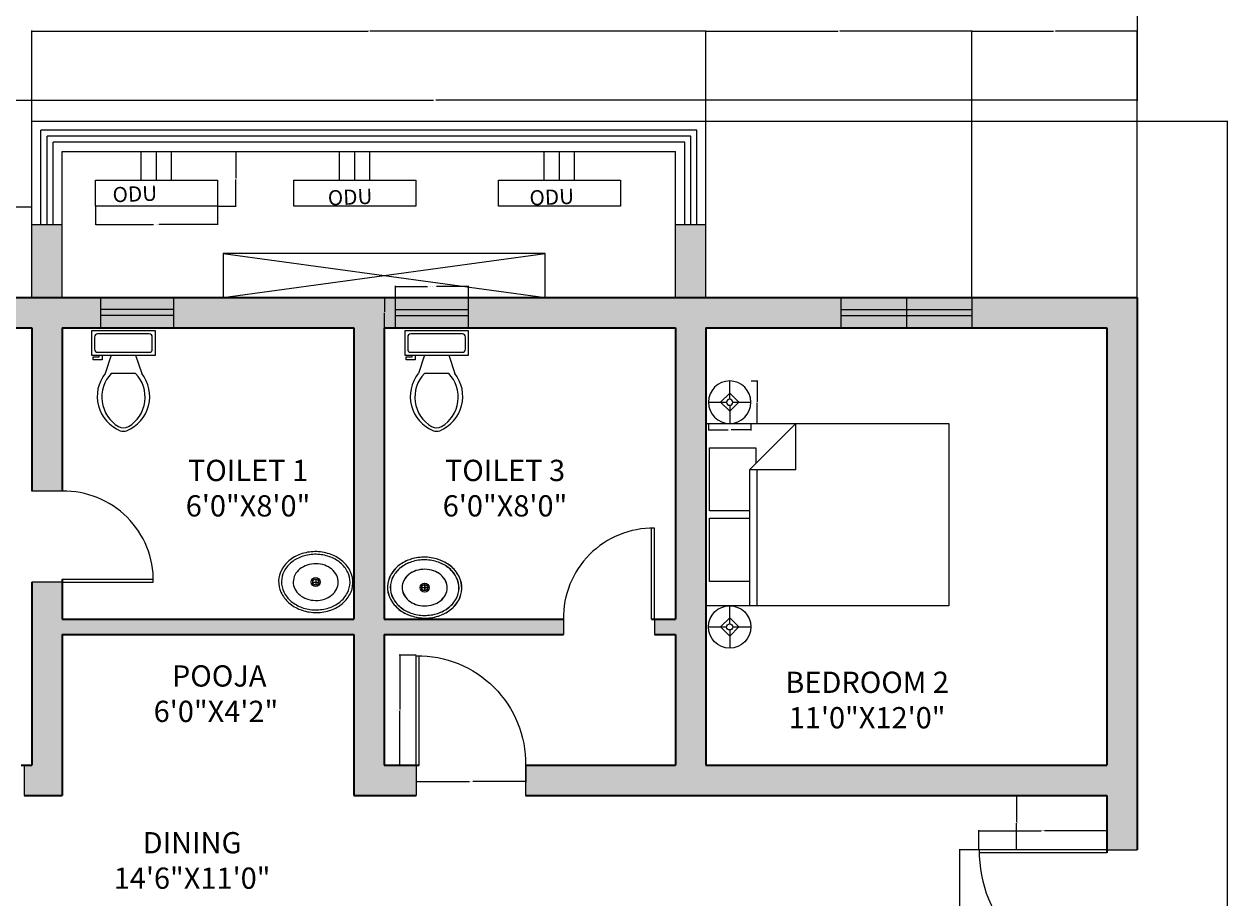
# Model space of a CAD drawing. Units: inches. Extents: x -382 to 250, y 518 to 1732.
# Tile 4 of 8: x -147 to 250, y 879 to 1167. Entities that reach past the tile are written whole.
import ezdxf

# ---------------------------------------------------------------- set-up
doc = ezdxf.new("R2010")
doc.units = ezdxf.units.IN
doc.header["$MEASUREMENT"] = 0
for name, color, linetype, lineweight in [('A-ANNO-DIMS', 2, 'Continuous', 18), ('A-AREA-IDEN', 7, 'Continuous', 18), ('A-DOOR', 3, 'Continuous', 18), ('A-FLOR-EDGE', 7, 'Continuous', 25), ('A-FLOR-FIXT', 8, 'Continuous', 18), ('A-FLOR-SHFT', 8, 'Continuous', 18), ('A-FURN', 8, 'Continuous', 18), ('A-GLAZ', 4, 'Continuous', 18), ('A-WALL', 7, 'Continuous', 35), ('M-ANNO-TEXT', 7, 'Continuous', 13), ('M-HVAC-EQPM', 4, 'Continuous', 18)]:
    doc.layers.add(name, color=color, linetype=linetype, lineweight=lineweight)
doc.layers.add('A-GLAZ-PATT', color=143, linetype='Continuous', lineweight=13, true_color=0x7aafdf)
doc.layers.add('A-WALL-PATT', color=251, linetype='Continuous', lineweight=13, true_color=0x636466)
doc.styles.get("Standard").update_dxf_attribs({"font": 'arial.ttf'})
doc.dimstyles.get("Standard").update_dxf_attribs({"dimtxt": 0.18, "dimasz": 0.18, "dimexe": 0.18, "dimexo": 0.0625, "dimgap": 0.09, "dimtad": 0, "dimtih": 1, "dimtoh": 1, "dimdec": 4, "dimzin": 0, "dimdsep": 46, "dimtxsty": 'Standard', "dimcen": 0.09, "dimadec": 0, "dimazin": 0, "dimtfac": 1, "dimtdec": 4, "dimtofl": 0, "dimtmove": 0, "dimatfit": 3, "dimfxl": 1, "dimtolj": 1, "dimtzin": 0, "dimarcsym": 0})

# ---------------------------------------------------------------- blocks, each defined once
blk = doc.blocks.new('Sink - Oval top')
for p, q in [((-1, 0), (1, 0)), ((0, 1), (0, -1))]:
    blk.add_line(p, q)
for points in [[(-12.23, 0.39, 0.117634), (-11.46, -3.36, 0.104469), (-8.88, -6.8, 0.090016), (-5.08, -9.07, 0.08192), (-0.32, -10.02, 0.08192), (4.49, -9.38, 0.090016), (8.42, -7.36, 0.104469), (11.22, -4.09, 0.117634), (12.23, -0.39, 0.117634), (11.46, 3.36, 0.104469), (8.88, 6.8, 0.090016), (5.08, 9.07, 0.08192), (0.32, 10.02, 0.08192), (-4.49, 9.38, 0.090016), (-8.42, 7.36, 0.104469), (-11.22, 4.09, 0.117634)], [(-11.29, 0.16, 0.118622), (-10.52, -3.25, 0.104678), (-8.07, -6.36, 0.089562), (-4.54, -8.37, 0.081185), (-0.13, -9.15, 0.081185), (4.3, -8.49, 0.089562), (7.89, -6.58, 0.104678), (10.42, -3.55, 0.118622), (11.29, -0.16, 0.118622), (10.52, 3.25, 0.104678), (8.07, 6.36, 0.089562), (4.54, 8.37, 0.081185), (0.13, 9.15, 0.081185), (-4.3, 8.49, 0.089562), (-7.89, 6.58, 0.104678), (-10.42, 3.55, 0.118622)], [(-7.42, 0.08, 0.118283), (-6.91, -2.17, 0.104607), (-5.29, -4.21, 0.089718), (-2.97, -5.53, 0.081436), (-0.07, -6.04, 0.081436), (2.84, -5.59, 0.089718), (5.2, -4.33, 0.104607), (6.86, -2.32, 0.118283), (7.42, -0.08, 0.118283), (6.91, 2.17, 0.104607), (5.29, 4.21, 0.089718), (2.97, 5.53, 0.081436), (0.07, 6.04, 0.081436), (-2.84, 5.59, 0.089718), (-5.2, 4.33, 0.104607), (-6.86, 2.32, 0.118283)]]:
    blk.add_lwpolyline(points, format="xyb", close=True)
for radius in [1.5, 1]:
    blk.add_circle((0, 0), radius)
blk = doc.blocks.new('Bed - Queen')
for p, q in [((0, -80.00003), (0, 0)), ((0, 0), (59.99999, 0)), ((59.99999, 0), (59.99999, -80.00003)), ((7.99999, -1.2), (28.79998, -1.2)), ((7.99999, -14.4), (7.99999, -1.2)), ((28.79998, -1.2), (28.79998, -14.4)), ((31.19999, -1.2), (51.99999, -1.2)), ((31.19999, -14.4), (31.19999, -1.2)), ((51.99999, -1.2), (51.99999, -16.4)), ((0, -14.4), (44.8, -14.4)), ((59.99999, -29.6), (44.8, -14.4)), ((44.8, -14.4), (44.8, -29.6)), ((44.8, -16.8), (0, -16.8)), ((51.99999, -16.4), (46.79936, -16.4)), ((44.8, -29.6), (59.99999, -29.6)), ((59.99999, -80.00003), (0, -80.00003))]:
    blk.add_line(p, q)
blk = doc.blocks.new('Lamp - Table')
for p, q in [((0, 7), (0, 1)), ((-1, 0), (-7, 0)), ((0, 3), (-3, 0)), ((-3, 0), (0, -3)), ((3, 0), (0, 3)), ((0, -3), (3, 0)), ((1, 0), (7, 0)), ((0, -1), (0, -7))]:
    blk.add_line(p, q)
for radius in [7, 1]:
    blk.add_circle((0, 0), radius)
blk = doc.blocks.new('Toilet - top')
for p, q in [((9.5, -6), (9.5, -2)), ((-10, -8.5), (-8, -8.5)), ((-10, -9.5), (-10, -8.5)), ((-7, -9.5), (-10, -9.5)), ((-8, -8.5), (-8, -8)), ((-7, -8), (-7, -9.5)), ((-4, -8), (-6, -14)), ((4, -8), (6, -14)), ((4, -14), (-4, -14))]:
    blk.add_line(p, q)
blk.add_lwpolyline([(10.5, -8), (10.5, 0), (-10.5, 0), (-10.5, -8)], close=True)
for points in [[(-9.5, -2), (-9.5, -6)], [(8.5, -1), (-8.5, -1)], [(-8.5, -7), (8.5, -7)]]:
    blk.add_lwpolyline(points)
for centre, radius, start, end in [((-8.62, -1.88), 0.884, 81.8699, 188.1301), ((8.62, -1.88), 0.884, 351.8699, 98.1301), ((-8.62, -6.12), 0.884, 171.8699, 278.1301), ((8.62, -6.12), 0.884, 261.8699, 8.1301), ((3.52, -21.58), 12.17, 141.4691, 247.9714), ((4.2, -21.82), 11.33, 136.3677, 238.9468), ((-3.52, -21.58), 12.17, 292.0284, 38.5307), ((-4.2, -21.82), 11.33, 301.053, 43.6321), ((0, -27.88), 4, 245.7318, 294.2682), ((0, -29), 4, 254.8605, 285.1395)]:
    blk.add_arc(centre, radius, start, end)
blk = doc.blocks.new('WIN-24IN')
for p, q in [((0, 0), (0, 10)), ((24, 0), (24, 10)), ((0, 6), (24, 6)), ((0, 4), (24, 4))]:
    blk.add_line(p, q)
blk = doc.blocks.new('DOOR-SWING-36IN')
for p, q in [((-1, 0), (-1, 36)), ((0, 0), (0, 36))]:
    blk.add_line(p, q)
blk.add_arc((-0.5, 0.5), 35.5, 89.1931, 180.8069)
blk = doc.blocks.new('DOOR-SWING-30IN')
for p, q in [((0, 1), (30, 1)), ((0, 0), (30, 0))]:
    blk.add_line(p, q)
blk.add_arc((0.5, 0.5), 29.5, 359.029, 90.971)
blk = doc.blocks.new('ODU-LEDGE-LARGE')
for p, q in [((15.1, 8.56), (15.1, 17.94)), ((20.1, 8.56), (20.1, 17.94)), ((25.1, 8.56), (25.1, 17.94))]:
    blk.add_line(p, q)
blk.add_lwpolyline([(0, 8.56), (40.21, 8.56), (40.21, 0), (0, 0)], close=True)
blk = doc.blocks.new('DOOR-ENTRY-42IN')
for p, q in [((0, 0), (-42, 0)), ((0, -1), (-42, -1))]:
    blk.add_line(p, q)
blk.add_arc((-0.5, -0.5), 41.5, 179.3097, 270.6903)
blk = doc.blocks.new('*D30')
at = {"layer": 'A-ANNO-DIMS', "color": 0, "lineweight": -2, "transparency": 16777216}
for p, q in [((92.66, 1049.55), (94.88, 1049.55)), ((94.7, 1049.37), (94.7, 1042.73)), ((94.7, 1035.73), (94.7, 1042.37)), ((92.66, 1035.55), (94.88, 1035.55))]:
    blk.add_line(p, q, dxfattribs=at)
at = {"layer": 'A-ANNO-DIMS', "color": 0, "transparency": 16777216}
for points in [[(94.67, 1049.37), (94.73, 1049.37), (94.7, 1049.55)], [(94.67, 1035.73), (94.73, 1035.73), (94.7, 1035.55)]]:
    blk.add_solid(points, dxfattribs=at)
at = {"layer": 'Defpoints', "color": 0, "transparency": 16777216}
for p in [(92.6, 1049.55), (92.6, 1035.55), (94.7, 1035.55)]:
    blk.add_point(p, dxfattribs=at)
at = {"layer": 'A-ANNO-DIMS', "color": 0, "transparency": 16777216, "insert": (94.7, 1042.55), "char_height": 0.18, "attachment_point": 5}
blk.add_mtext('\\A1;LAMP 14 TYP.', dxfattribs=at)
blk = doc.blocks.new('*D31')
at = {"layer": 'A-ANNO-DIMS', "color": 0, "lineweight": -2, "transparency": 16777216}
for p, q in [((78.6, 1035.49), (78.6, 1033.27)), ((92.6, 1035.49), (92.6, 1033.27)), ((78.78, 1033.45), (85.08, 1033.45)), ((92.42, 1033.45), (86.12, 1033.45))]:
    blk.add_line(p, q, dxfattribs=at)
at = {"layer": 'A-ANNO-DIMS', "color": 0, "transparency": 16777216}
for points in [[(78.78, 1033.48), (78.78, 1033.42), (78.6, 1033.45)], [(92.42, 1033.48), (92.42, 1033.42), (92.6, 1033.45)]]:
    blk.add_solid(points, dxfattribs=at)
at = {"layer": 'Defpoints', "color": 0, "transparency": 16777216}
for p in [(78.6, 1035.55), (92.6, 1035.55), (78.6, 1033.45)]:
    blk.add_point(p, dxfattribs=at)
at = {"layer": 'A-ANNO-DIMS', "color": 0, "transparency": 16777216, "insert": (85.6, 1033.45), "char_height": 0.18, "attachment_point": 5}
blk.add_mtext('\\A1;14 TYP.', dxfattribs=at)
blk = doc.blocks.new('*D50')
at = {"layer": 'A-ANNO-DIMS', "color": 0, "lineweight": -2, "transparency": 16777216}
for p, q in [((-123.3, 1107.06), (-123.3, 1100.92)), ((-83.09, 1107.06), (-83.09, 1100.92)), ((-123.12, 1101.1), (-104.15, 1101.1)), ((-83.27, 1101.1), (-102.24, 1101.1))]:
    blk.add_line(p, q, dxfattribs=at)
at = {"layer": 'A-ANNO-DIMS', "color": 0, "transparency": 16777216}
for points in [[(-123.12, 1101.13), (-123.12, 1101.07), (-123.3, 1101.1)], [(-83.27, 1101.13), (-83.27, 1101.07), (-83.09, 1101.1)]]:
    blk.add_solid(points, dxfattribs=at)
at = {"layer": 'Defpoints', "color": 0, "transparency": 16777216}
for p in [(-123.3, 1107.13), (-83.09, 1107.13), (-83.09, 1101.1)]:
    blk.add_point(p, dxfattribs=at)
at = {"layer": 'A-ANNO-DIMS', "color": 0, "transparency": 16777216, "insert": (-103.2, 1101.1), "char_height": 0.18, "attachment_point": 5}
blk.add_mtext('\\A1;ODU-L 40 TYP.', dxfattribs=at)
blk = doc.blocks.new('*D51')
at = {"layer": 'A-ANNO-DIMS', "color": 0, "lineweight": -2, "transparency": 16777216}
for p, q in [((-83.03, 1125.07), (-76.88, 1125.07)), ((-77.06, 1124.89), (-77.06, 1116.28)), ((-77.06, 1107.31), (-77.06, 1115.92)), ((-83.03, 1107.13), (-76.88, 1107.13))]:
    blk.add_line(p, q, dxfattribs=at)
at = {"layer": 'A-ANNO-DIMS', "color": 0, "transparency": 16777216}
for points in [[(-77.09, 1124.89), (-77.03, 1124.89), (-77.06, 1125.07)], [(-77.09, 1107.31), (-77.03, 1107.31), (-77.06, 1107.13)]]:
    blk.add_solid(points, dxfattribs=at)
at = {"layer": 'Defpoints', "color": 0, "transparency": 16777216}
for p in [(-83.09, 1125.07), (-77.06, 1125.07), (-83.09, 1107.13)]:
    blk.add_point(p, dxfattribs=at)
at = {"layer": 'A-ANNO-DIMS', "color": 0, "transparency": 16777216, "insert": (-77.06, 1116.1), "char_height": 0.18, "attachment_point": 5}
blk.add_mtext('\\A1;18 TYP.', dxfattribs=at)
blk = doc.blocks.new('*D58')
at = {"layer": 'A-ANNO-DIMS', "color": 0, "lineweight": -2, "transparency": 16777216}
for p, q in [((167.59, 895.12), (161.15, 895.12)), ((161.33, 894.94), (161.33, 874.24)), ((161.33, 853.17), (161.33, 873.87)), ((167.59, 852.99), (161.15, 852.99))]:
    blk.add_line(p, q, dxfattribs=at)
at = {"layer": 'A-ANNO-DIMS', "color": 0, "transparency": 16777216}
for points in [[(161.3, 894.94), (161.36, 894.94), (161.33, 895.12)], [(161.3, 853.17), (161.36, 853.17), (161.33, 852.99)]]:
    blk.add_solid(points, dxfattribs=at)
at = {"layer": 'Defpoints', "color": 0, "transparency": 16777216}
for p in [(161.33, 895.12), (167.65, 895.12), (167.65, 852.99)]:
    blk.add_point(p, dxfattribs=at)
at = {"layer": 'A-ANNO-DIMS', "color": 0, "transparency": 16777216, "insert": (161.33, 874.06), "char_height": 0.18, "attachment_point": 5}
blk.add_mtext('\\A1;ENTRY DOOR 42 TYP.', dxfattribs=at)
blk = doc.blocks.new('*D59')
at = {"layer": 'A-ANNO-DIMS', "color": 0, "lineweight": -2, "transparency": 16777216}
for p, q in [((167.65, 895.19), (167.65, 901.62)), ((167.83, 901.44), (188.19, 901.44)), ((209.6, 901.44), (189.25, 901.44)), ((209.78, 895.19), (209.78, 901.62))]:
    blk.add_line(p, q, dxfattribs=at)
at = {"layer": 'A-ANNO-DIMS', "color": 0, "transparency": 16777216}
for points in [[(167.83, 901.47), (167.83, 901.41), (167.65, 901.44)], [(209.6, 901.47), (209.6, 901.41), (209.78, 901.44)]]:
    blk.add_solid(points, dxfattribs=at)
at = {"layer": 'Defpoints', "color": 0, "transparency": 16777216}
for p in [(209.78, 901.44), (167.65, 895.12), (209.78, 895.12)]:
    blk.add_point(p, dxfattribs=at)
at = {"layer": 'A-ANNO-DIMS', "color": 0, "transparency": 16777216, "insert": (188.72, 901.44), "char_height": 0.18, "attachment_point": 5}
blk.add_mtext('\\A1;42 TYP.', dxfattribs=at)
blk = doc.blocks.new('*D60')
at = {"layer": 'A-ANNO-DIMS', "color": 0, "lineweight": -2, "transparency": 16777216}
for p, q in [((-17.69, 959.2), (-23.22, 959.2)), ((-23.04, 959.02), (-23.04, 941.32)), ((-23.04, 923.25), (-23.04, 940.95)), ((-17.69, 923.07), (-23.22, 923.07))]:
    blk.add_line(p, q, dxfattribs=at)
at = {"layer": 'A-ANNO-DIMS', "color": 0, "transparency": 16777216}
for points in [[(-23.07, 959.02), (-23.01, 959.02), (-23.04, 959.2)], [(-23.07, 923.25), (-23.01, 923.25), (-23.04, 923.07)]]:
    blk.add_solid(points, dxfattribs=at)
at = {"layer": 'Defpoints', "color": 0, "transparency": 16777216}
for p in [(-23.04, 959.2), (-17.62, 959.2), (-17.62, 923.07)]:
    blk.add_point(p, dxfattribs=at)
at = {"layer": 'A-ANNO-DIMS', "color": 0, "transparency": 16777216, "insert": (-23.04, 941.14), "char_height": 0.18, "attachment_point": 5}
blk.add_mtext('\\A1;ROOM DOOR 36 TYP.', dxfattribs=at)
blk = doc.blocks.new('*D61')
at = {"layer": 'A-ANNO-DIMS', "color": 0, "lineweight": -2, "transparency": 16777216}
for p, q in [((-17.62, 923.01), (-17.62, 917.47)), ((18.51, 923.01), (18.51, 917.47)), ((-17.44, 917.65), (-0.08, 917.65)), ((18.33, 917.65), (0.97, 917.65))]:
    blk.add_line(p, q, dxfattribs=at)
at = {"layer": 'A-ANNO-DIMS', "color": 0, "transparency": 16777216}
for points in [[(-17.44, 917.68), (-17.44, 917.62), (-17.62, 917.65)], [(18.33, 917.68), (18.33, 917.62), (18.51, 917.65)]]:
    blk.add_solid(points, dxfattribs=at)
at = {"layer": 'Defpoints', "color": 0, "transparency": 16777216}
for p in [(-17.62, 923.07), (18.51, 923.07), (-17.62, 917.65)]:
    blk.add_point(p, dxfattribs=at)
at = {"layer": 'A-ANNO-DIMS', "color": 0, "transparency": 16777216, "insert": (0.44, 917.65), "char_height": 0.18, "attachment_point": 5}
blk.add_mtext('\\A1;36 TYP.', dxfattribs=at)
blk = doc.blocks.new('*D72')
at = {"layer": 'A-ANNO-DIMS', "color": 0, "lineweight": -2, "transparency": 16777216}
for p, q in [((-24.44, 1077.13), (-24.44, 1080.85)), ((-24.26, 1080.67), (-13.93, 1080.67)), ((-0.62, 1080.67), (-10.95, 1080.67)), ((-0.44, 1077.13), (-0.44, 1080.85))]:
    blk.add_line(p, q, dxfattribs=at)
at = {"layer": 'A-ANNO-DIMS', "color": 0, "transparency": 16777216}
for points in [[(-24.26, 1080.7), (-24.26, 1080.64), (-24.44, 1080.67)], [(-0.62, 1080.7), (-0.62, 1080.64), (-0.44, 1080.67)]]:
    blk.add_solid(points, dxfattribs=at)
at = {"layer": 'Defpoints', "color": 0, "transparency": 16777216}
for p in [(-0.44, 1080.67), (-24.44, 1077.07), (-0.44, 1077.07)]:
    blk.add_point(p, dxfattribs=at)
at = {"layer": 'A-ANNO-DIMS', "color": 0, "transparency": 16777216, "insert": (-12.44, 1080.67), "char_height": 0.18, "attachment_point": 5}
blk.add_mtext('\\A1;VENT WINDOW 24 TYP.', dxfattribs=at)
blk = doc.blocks.new('*D73')
at = {"layer": 'A-ANNO-DIMS', "color": 0, "lineweight": -2, "transparency": 16777216}
for p, q in [((-24.5, 1077.07), (-28.22, 1077.07)), ((-28.04, 1076.89), (-28.04, 1072.25)), ((-28.04, 1067.25), (-28.04, 1071.89)), ((-24.5, 1067.07), (-28.22, 1067.07))]:
    blk.add_line(p, q, dxfattribs=at)
at = {"layer": 'A-ANNO-DIMS', "color": 0, "transparency": 16777216}
for points in [[(-28.07, 1076.89), (-28.01, 1076.89), (-28.04, 1077.07)], [(-28.07, 1067.25), (-28.01, 1067.25), (-28.04, 1067.07)]]:
    blk.add_solid(points, dxfattribs=at)
at = {"layer": 'Defpoints', "color": 0, "transparency": 16777216}
for p in [(-28.04, 1077.07), (-24.44, 1077.07), (-24.44, 1067.07)]:
    blk.add_point(p, dxfattribs=at)
at = {"layer": 'A-ANNO-DIMS', "color": 0, "transparency": 16777216, "insert": (-28.04, 1072.07), "char_height": 0.18, "attachment_point": 5}
blk.add_mtext('\\A1;10 TYP.', dxfattribs=at)
blk = doc.blocks.new('*D75')
at = {"layer": 'A-ANNO-DIMS', "color": 0, "lineweight": -2, "transparency": 16777216}
for p, q in [((77.85, 1135.07), (249.66, 1135.07)), ((249.48, 1134.89), (249.48, 841.75)), ((249.48, 548.25), (249.48, 841.39)), ((58.85, 548.07), (249.66, 548.07))]:
    blk.add_line(p, q, dxfattribs=at)
at = {"layer": 'A-ANNO-DIMS', "color": 0, "transparency": 16777216}
for points in [[(249.45, 1134.89), (249.51, 1134.89), (249.48, 1135.07)], [(249.45, 548.25), (249.51, 548.25), (249.48, 548.07)]]:
    blk.add_solid(points, dxfattribs=at)
at = {"layer": 'Defpoints', "color": 0, "transparency": 16777216}
for p in [(77.78, 1135.07), (249.48, 1135.07), (58.78, 548.07)]:
    blk.add_point(p, dxfattribs=at)
at = {"layer": 'A-ANNO-DIMS', "color": 0, "transparency": 16777216, "insert": (249.48, 841.57), "char_height": 0.18, "attachment_point": 5}
blk.add_mtext('\\A1;587', dxfattribs=at)
blk = doc.blocks.new('*D76')
at = {"layer": 'A-ANNO-DIMS', "color": 0, "lineweight": -2, "transparency": 16777216}
for p, q in [((-298.22, 1077.13), (-298.22, 1106.95)), ((-298.04, 1106.77), (-221.5, 1106.77)), ((-144.4, 1106.77), (-220.94, 1106.77)), ((-144.22, 1077.13), (-144.22, 1106.95))]:
    blk.add_line(p, q, dxfattribs=at)
at = {"layer": 'A-ANNO-DIMS', "color": 0, "transparency": 16777216}
for points in [[(-298.04, 1106.8), (-298.04, 1106.74), (-298.22, 1106.77)], [(-144.4, 1106.8), (-144.4, 1106.74), (-144.22, 1106.77)]]:
    blk.add_solid(points, dxfattribs=at)
at = {"layer": 'Defpoints', "color": 0, "transparency": 16777216}
for p in [(-144.22, 1106.77), (-298.22, 1077.07), (-144.22, 1077.07)]:
    blk.add_point(p, dxfattribs=at)
at = {"layer": 'A-ANNO-DIMS', "color": 0, "transparency": 16777216, "insert": (-221.22, 1106.77), "char_height": 0.18, "attachment_point": 5}
blk.add_mtext('\\A1;154', dxfattribs=at)
blk = doc.blocks.new('*D77')
at = {"layer": 'A-ANNO-DIMS', "color": 0, "lineweight": -2, "transparency": 16777216}
for p, q in [((-144.22, 1135.13), (-144.22, 1164.95)), ((-144.04, 1164.77), (-33.5, 1164.77)), ((77.6, 1164.77), (-32.93, 1164.77)), ((77.78, 1135.13), (77.78, 1164.95))]:
    blk.add_line(p, q, dxfattribs=at)
at = {"layer": 'A-ANNO-DIMS', "color": 0, "transparency": 16777216}
for points in [[(-144.04, 1164.8), (-144.04, 1164.74), (-144.22, 1164.77)], [(77.6, 1164.8), (77.6, 1164.74), (77.78, 1164.77)]]:
    blk.add_solid(points, dxfattribs=at)
at = {"layer": 'Defpoints', "color": 0, "transparency": 16777216}
for p in [(77.78, 1164.77), (-144.22, 1135.07), (77.78, 1135.07)]:
    blk.add_point(p, dxfattribs=at)
at = {"layer": 'A-ANNO-DIMS', "color": 0, "transparency": 16777216, "insert": (-33.22, 1164.77), "char_height": 0.18, "attachment_point": 5}
blk.add_mtext('\\A1;222', dxfattribs=at)
blk = doc.blocks.new('*D78')
at = {"layer": 'A-ANNO-DIMS', "color": 0, "lineweight": -2, "transparency": 16777216}
for p, q in [((77.78, 1135.13), (77.78, 1164.95)), ((77.96, 1164.77), (121.26, 1164.77)), ((165.2, 1164.77), (121.91, 1164.77)), ((165.38, 1077.13), (165.38, 1164.95))]:
    blk.add_line(p, q, dxfattribs=at)
at = {"layer": 'A-ANNO-DIMS', "color": 0, "transparency": 16777216}
for points in [[(77.96, 1164.8), (77.96, 1164.74), (77.78, 1164.77)], [(165.2, 1164.8), (165.2, 1164.74), (165.38, 1164.77)]]:
    blk.add_solid(points, dxfattribs=at)
at = {"layer": 'Defpoints', "color": 0, "transparency": 16777216}
for p in [(165.38, 1164.77), (77.78, 1135.07), (165.38, 1077.07)]:
    blk.add_point(p, dxfattribs=at)
at = {"layer": 'A-ANNO-DIMS', "color": 0, "transparency": 16777216, "insert": (121.58, 1164.77), "char_height": 0.18, "attachment_point": 5}
blk.add_mtext('\\A1;87.6', dxfattribs=at)
blk = doc.blocks.new('*D83')
at = {"layer": 'A-ANNO-DIMS', "color": 0, "lineweight": -2, "transparency": 16777216}
for p, q in [((209.72, 913.07), (179.9, 913.07)), ((180.08, 912.89), (180.08, 904.28)), ((180.08, 895.3), (180.08, 903.91)), ((209.72, 895.12), (179.9, 895.12))]:
    blk.add_line(p, q, dxfattribs=at)
at = {"layer": 'A-ANNO-DIMS', "color": 0, "transparency": 16777216}
for points in [[(180.05, 912.89), (180.11, 912.89), (180.08, 913.07)], [(180.05, 895.3), (180.11, 895.3), (180.08, 895.12)]]:
    blk.add_solid(points, dxfattribs=at)
at = {"layer": 'Defpoints', "color": 0, "transparency": 16777216}
for p in [(180.08, 913.07), (209.78, 913.07), (209.78, 895.12)]:
    blk.add_point(p, dxfattribs=at)
at = {"layer": 'A-ANNO-DIMS', "color": 0, "transparency": 16777216, "insert": (180.08, 904.1), "char_height": 0.18, "attachment_point": 5}
blk.add_mtext('\\A1;17.945', dxfattribs=at)
blk = doc.blocks.new('*D84')
at = {"layer": 'A-ANNO-DIMS', "color": 0, "lineweight": -2, "transparency": 16777216}
for p, q in [((165.38, 1077.13), (165.38, 1164.95)), ((165.56, 1164.77), (192.26, 1164.77)), ((219.6, 1164.77), (192.91, 1164.77)), ((219.78, 1077.13), (219.78, 1164.95))]:
    blk.add_line(p, q, dxfattribs=at)
at = {"layer": 'A-ANNO-DIMS', "color": 0, "transparency": 16777216}
for points in [[(165.56, 1164.8), (165.56, 1164.74), (165.38, 1164.77)], [(219.6, 1164.8), (219.6, 1164.74), (219.78, 1164.77)]]:
    blk.add_solid(points, dxfattribs=at)
at = {"layer": 'Defpoints', "color": 0, "transparency": 16777216}
for p in [(219.78, 1164.77), (165.38, 1077.07), (219.78, 1077.07)]:
    blk.add_point(p, dxfattribs=at)
at = {"layer": 'A-ANNO-DIMS', "color": 0, "transparency": 16777216, "insert": (192.58, 1164.77), "char_height": 0.18, "attachment_point": 5}
blk.add_mtext('\\A1;54.4', dxfattribs=at)
blk = doc.blocks.new('*D86')
at = {"layer": 'A-ANNO-DIMS', "color": 0, "lineweight": -2, "transparency": 16777216}
for p, q in [((-242.98, 1352.01), (-242.98, 1141.82)), ((219.78, 1197.01), (219.78, 1141.82)), ((-242.8, 1142), (-11.99, 1142)), ((219.6, 1142), (-11.2, 1142))]:
    blk.add_line(p, q, dxfattribs=at)
at = {"layer": 'A-ANNO-DIMS', "color": 0, "transparency": 16777216}
for points in [[(-242.8, 1142.03), (-242.8, 1141.97), (-242.98, 1142)], [(219.6, 1142.03), (219.6, 1141.97), (219.78, 1142)]]:
    blk.add_solid(points, dxfattribs=at)
at = {"layer": 'Defpoints', "color": 0, "transparency": 16777216}
for p in [(-242.98, 1352.07), (219.78, 1197.07), (219.78, 1142)]:
    blk.add_point(p, dxfattribs=at)
at = {"layer": 'A-ANNO-DIMS', "color": 0, "transparency": 16777216, "insert": (-11.6, 1142), "char_height": 0.18, "attachment_point": 5}
blk.add_mtext('\\A1;462.8', dxfattribs=at)

msp = doc.modelspace()

# ---------------------------------------------------------------- hatches: boundary and pattern name
at = {"layer": 'A-GLAZ-PATT'}
h = msp.add_hatch(color=256, dxfattribs=at)
h.dxf.hatch_style = 1
h.paths.add_polyline_path([(-97.6147, 1077.0687), (-121.6147, 1077.0687), (-121.6147, 1073.0687), (-97.6147, 1073.0687)])
h = msp.add_hatch(color=256, dxfattribs=at)
h.dxf.hatch_style = 1
h.paths.add_polyline_path([(-0.4384, 1077.0687), (-24.4384, 1077.0687), (-24.4384, 1073.0687), (-0.4384, 1073.0687)])
h = msp.add_hatch(color=256, dxfattribs=at)
h.dxf.hatch_style = 1
h.paths.add_polyline_path([(143.785, 1077.0687), (122.185, 1077.0687), (122.185, 1073.0687), (143.785, 1073.0687)])
h = msp.add_hatch(color=256, dxfattribs=at)
h.dxf.hatch_style = 1
h.paths.add_polyline_path([(165.385, 1077.0687), (143.785, 1077.0687), (143.785, 1073.0687), (165.385, 1073.0687)])
h = msp.add_hatch(color=256, dxfattribs=at)
h.dxf.hatch_style = 1
h.paths.add_polyline_path([(-97.6147, 1073.0687), (-121.6147, 1073.0687), (-121.6147, 1071.0687), (-97.6147, 1071.0687)])
h = msp.add_hatch(color=256, dxfattribs=at)
h.dxf.hatch_style = 1
h.paths.add_polyline_path([(-97.6147, 1071.0687), (-121.6147, 1071.0687), (-121.6147, 1067.0687), (-97.6147, 1067.0687)])
h = msp.add_hatch(color=256, dxfattribs=at)
h.dxf.hatch_style = 1
h.paths.add_polyline_path([(-0.4384, 1073.0687), (-24.4384, 1073.0687), (-24.4384, 1071.0687), (-0.4384, 1071.0687)])
h = msp.add_hatch(color=256, dxfattribs=at)
h.dxf.hatch_style = 1
h.paths.add_polyline_path([(-0.4384, 1071.0687), (-24.4384, 1071.0687), (-24.4384, 1067.0687), (-0.4384, 1067.0687)])
h = msp.add_hatch(color=256, dxfattribs=at)
h.dxf.hatch_style = 1
h.paths.add_polyline_path([(143.785, 1073.0687), (122.185, 1073.0687), (122.185, 1071.0687), (143.785, 1071.0687)])
h = msp.add_hatch(color=256, dxfattribs=at)
h.dxf.hatch_style = 1
h.paths.add_polyline_path([(143.785, 1071.0687), (122.185, 1071.0687), (122.185, 1067.0687), (143.785, 1067.0687)])
h = msp.add_hatch(color=256, dxfattribs=at)
h.dxf.hatch_style = 1
h.paths.add_polyline_path([(165.385, 1073.0687), (143.785, 1073.0687), (143.785, 1071.0687), (165.385, 1071.0687)])
h = msp.add_hatch(color=256, dxfattribs=at)
h.dxf.hatch_style = 1
h.paths.add_polyline_path([(165.385, 1071.0687), (143.785, 1071.0687), (143.785, 1067.0687), (165.385, 1067.0687)])
at = {"layer": 'A-WALL-PATT'}
h = msp.add_hatch(color=256, dxfattribs=at)
h.dxf.hatch_style = 1
h.paths.add_polyline_path([(-134.215, 1101.0687), (-144.215, 1101.0687), (-144.215, 1077.0687), (-134.215, 1077.0687)])
h = msp.add_hatch(color=256, dxfattribs=at)
h.dxf.hatch_style = 1
h.paths.add_polyline_path([(77.785, 1101.0687), (67.785, 1101.0687), (67.785, 1077.0687), (77.785, 1077.0687)])
h = msp.add_hatch(color=256, dxfattribs=at)
h.dxf.hatch_style = 1
h.paths.add_polyline_path([(-121.6147, 1067.0687), (-121.6147, 1077.0687), (-194.615, 1077.0687), (-194.615, 1067.0687), (-144.215, 1067.0687), (-144.215, 1013.2912), (-134.215, 1013.2912), (-134.215, 1067.0687)])
h.paths.add_polyline_path([(-24.4384, 1067.0687), (-24.4384, 1077.0687), (-97.6147, 1077.0687), (-97.6147, 1067.0687), (-38.215, 1067.0687), (-38.215, 971.0687), (-134.215, 971.0687), (-134.215, 983.2912), (-144.215, 983.2912), (-144.215, 923.0687), (-146.7819, 923.0687), (-146.7819, 913.0687), (-134.215, 913.0687), (-134.215, 966.0687), (-38.215, 966.0687), (-38.215, 913.0687), (-28.215, 913.0687), (-17.6234, 913.0687), (-17.6234, 923.0687), (-28.215, 923.0687), (-28.215, 966.0687), (30.8449, 966.0687), (30.8449, 971.0687), (-28.215, 971.0687), (-28.215, 1067.0687)])
h.paths.add_polyline_path([(-0.4384, 1077.0687), (-0.4384, 1067.0687), (67.785, 1067.0687), (67.785, 971.0687), (60.8449, 971.0687), (60.8449, 966.0687), (67.785, 966.0687), (67.785, 923.0687), (18.3766, 923.0687), (18.3766, 913.0687), (209.785, 913.0687), (209.785, 895.1233), (219.785, 895.1233), (219.785, 913.0687), (219.785, 1077.0687), (165.385, 1077.0687), (165.385, 1067.0687), (209.785, 1067.0687), (209.785, 923.0687), (77.785, 923.0687), (77.785, 1067.0687), (122.185, 1067.0687), (122.185, 1077.0687)])

# ---------------------------------------------------------------- linework, layer by layer
at = {"layer": 'A-DOOR'}
for p, q in [((-134.215, 1013.2912), (-144.215, 1013.2912)), ((-134.215, 983.2912), (-144.215, 983.2912)), ((30.8449, 971.0687), (30.8449, 966.0687)), ((60.8449, 971.0687), (60.8449, 966.0687)), ((-146.7819, 923.0687), (-146.7819, 913.0687)), ((-17.6234, 923.0687), (-17.6234, 913.0687)), ((18.3766, 923.0687), (18.3766, 913.0687)), ((209.785, 895.1233), (219.785, 895.1233))]:
    msp.add_line(p, q, dxfattribs=at)
at = {"layer": 'A-FLOR-EDGE'}
for p, q in [((-144.215, 1077.0687), (-144.215, 1135.0687)), ((-144.215, 1135.0687), (77.785, 1135.0687)), ((77.785, 1077.0687), (77.785, 1135.0687)), ((74.785, 1132.1839), (-141.215, 1132.1839)), ((-141.215, 1101.0687), (-141.215, 1132.1839)), ((-139.215, 1101.0687), (-139.215, 1130.1839)), ((72.785, 1130.1839), (-139.215, 1130.1839)), ((72.785, 1101.0687), (72.785, 1130.1839)), ((74.785, 1101.0687), (74.785, 1132.1839)), ((70.785, 1128.1839), (-137.215, 1128.1839)), ((-137.215, 1101.0687), (-137.215, 1128.1839)), ((70.785, 1101.0687), (70.785, 1128.1839)), ((-134.215, 1077.0687), (-134.215, 1125.0687)), ((-134.215, 1125.0687), (67.785, 1125.0687)), ((67.785, 1077.0687), (67.785, 1125.0687)), ((-144.215, 1101.0687), (-134.215, 1101.0687)), ((67.785, 1101.0687), (77.785, 1101.0687))]:
    msp.add_line(p, q, dxfattribs=at)
at = {"layer": 'A-FLOR-SHFT'}
for p, q in [((-81.215, 1077.0687), (24.785, 1091.5188)), ((-81.215, 1091.5188), (24.785, 1077.0687))]:
    msp.add_line(p, q, dxfattribs=at)
msp.add_lwpolyline([(-81.215, 1077.0687), (24.785, 1077.0687), (24.785, 1091.5188), (-81.215, 1091.5188)], close=True, dxfattribs=at)
at = {"layer": 'A-GLAZ'}
for p, q in [((122.185, 1077.0687), (122.185, 1067.0687)), ((143.785, 1077.0687), (143.785, 1067.0687)), ((165.385, 1077.0687), (165.385, 1067.0687)), ((122.185, 1073.0687), (165.385, 1073.0687)), ((122.185, 1071.0687), (165.385, 1071.0687))]:
    msp.add_line(p, q, dxfattribs=at)
at = {"layer": 'A-WALL'}
for p, q in [((-298.215, 1077.0687), (-134.215, 1077.0687)), ((-134.215, 1077.0687), (-28.215, 1077.0687)), ((-28.215, 1077.0687), (77.785, 1077.0687)), ((77.785, 1077.0687), (219.785, 1077.0687)), ((219.785, 1077.0687), (219.785, 913.0687)), ((-288.215, 1067.0687), (-144.215, 1067.0687)), ((-144.215, 1067.0687), (-144.215, 1013.2912)), ((-134.215, 1067.0687), (-134.215, 1013.2912)), ((-134.215, 1067.0687), (-38.215, 1067.0687)), ((-38.215, 1067.0687), (-38.215, 971.0687)), ((-28.215, 1067.0687), (-28.215, 971.0687)), ((-28.215, 1067.0687), (67.785, 1067.0687)), ((67.785, 1067.0687), (67.785, 971.0687)), ((77.785, 1067.0687), (77.785, 923.0687)), ((77.785, 1067.0687), (209.785, 1067.0687)), ((209.785, 1067.0687), (209.785, 923.0687)), ((-144.215, 983.2912), (-144.215, 923.0687)), ((-134.215, 984.2912), (-134.215, 971.0687)), ((-134.215, 971.0687), (-38.215, 971.0687)), ((-28.215, 971.0687), (30.8449, 971.0687)), ((59.8449, 971.0687), (67.785, 971.0687)), ((-134.215, 966.0687), (-134.215, 913.0687)), ((-134.215, 966.0687), (-38.215, 966.0687)), ((-38.215, 966.0687), (-38.215, 913.0687)), ((-28.215, 966.0687), (-28.215, 923.0687)), ((-28.215, 966.0687), (30.8449, 966.0687)), ((60.8449, 966.0687), (67.785, 966.0687)), ((67.785, 966.0687), (67.785, 923.0687)), ((-147.7819, 923.0687), (-144.215, 923.0687)), ((-28.215, 923.0687), (-16.6234, 923.0687)), ((18.3766, 923.0687), (67.785, 923.0687)), ((77.785, 923.0687), (209.785, 923.0687)), ((-146.7819, 913.0687), (-134.215, 913.0687)), ((-38.215, 913.0687), (-28.215, 913.0687)), ((-28.215, 913.0687), (-17.6234, 913.0687)), ((18.3766, 913.0687), (209.785, 913.0687)), ((209.785, 913.0687), (209.785, 894.1233)), ((219.785, 913.0687), (219.785, 895.1233))]:
    msp.add_line(p, q, dxfattribs=at)
at = {"layer": 'M-HVAC-EQPM'}
msp.add_lwpolyline([(-57.9637, 1115.6904), (-17.7564, 1115.6904), (-17.7564, 1107.127), (-57.9637, 1107.127)], close=True, dxfattribs=at)

# ---------------------------------------------------------------- block references
at = {"layer": 'A-DOOR'}
for name, p in [('DOOR-SWING-30IN', (-134.215, 983.2912)), ('DOOR-ENTRY-42IN', (209.785, 895.1233))]:
    msp.add_blockref(name, p, dxfattribs=at)
at = {"layer": 'A-DOOR', "rotation": 90.00000000000031}
msp.add_blockref('DOOR-SWING-30IN', (60.8449, 971.0687), dxfattribs=at)
at = {"layer": 'A-DOOR', "extrusion": (0, 0, -1), "zscale": -1}
msp.add_blockref('DOOR-SWING-36IN', (17.6234, 923.0687), dxfattribs=at)
at = {"layer": 'A-FLOR-FIXT'}
for name, p in [('Toilet - top', (-114.0494, 1066.0319)), ('Toilet - top', (-10.9384, 1066.0319)), ('Sink - Oval top', (-50.7225, 983.3178)), ('Sink - Oval top', (-14.8728, 981.4966)), ('Sink - Oval top', (-14.835, 981.4966))]:
    msp.add_blockref(name, p, dxfattribs=at)
at = {"layer": 'A-FURN', "xscale": -1, "rotation": 90}
msp.add_blockref('Lamp - Table', (85.5964, 1042.5509), dxfattribs=at)
at = {"layer": 'A-FURN', "rotation": 90}
for name, p in [('Bed - Queen', (77.785, 975.5509)), ('Lamp - Table', (85.5964, 968.5509))]:
    msp.add_blockref(name, p, dxfattribs=at)
at = {"layer": 'A-GLAZ', "rotation": 180}
msp.add_blockref('WIN-24IN', (-97.6151, 1077.0684), dxfattribs=at)
at = {"layer": 'A-GLAZ'}
msp.add_blockref('WIN-24IN', (-24.438, 1067.069), dxfattribs=at)
at = {"layer": 'M-HVAC-EQPM'}
for p in [(-123.301, 1107.127), (-57.9641, 1107.127), (9.4423, 1107.127)]:
    msp.add_blockref('ODU-LEDGE-LARGE', p, dxfattribs=at)

# ---------------------------------------------------------------- texts
at = {"layer": 'A-AREA-IDEN', "char_height": 7, "attachment_point": 1}
for s, insert in [('\\pxqc;TOILET 1\\P6\'0"X8\'0"', (-112.8524, 1023.5927)), ('\\pxqc;TOILET 3\\P6\'0"X8\'0"', (-28.215, 1023.5927)), ('\\pxqc; POOJA\\P6\'0"X4\'2"', (-123.4182, 955.9115)), ('\\pxqc;BEDROOM 2\\P11\'0"X12\'0"', (91.0359, 953.8219)), ('\\pxqc;DINING\\P14\'6"X11\'0"', (-131.2791, 900.9865))]:
    msp.add_mtext_dynamic_manual_height_columns(s, width=79.656175, gutter_width=1, heights=[0], dxfattribs=dict(at, insert=insert))
at = {"layer": 'M-ANNO-TEXT', "char_height": 5, "attachment_point": 1, "rotation": 2.33497}
for insert in [(-117.7401, 1113.3453), (-46.8475, 1112.2967), (19.5636, 1112.2967)]:
    msp.add_mtext_dynamic_manual_height_columns('ODU', width=13.648337, gutter_width=1, heights=[0], dxfattribs=dict(at, insert=insert))

# ---------------------------------------------------------------- dimensions: what is measured, and where the dimension line sits
at = {"layer": 'A-ANNO-DIMS'}
for base, p1, p2, override, picture, middle in [((219.785, 1141.9977), (-242.9787, 1352.0687), (219.785, 1197.0687), {"dimdec": 1, "dimlfac": 1, "dimrnd": 0, "dimzin": 0, "dimdsep": 46, "dimlunit": 2}, '*D86', (-11.5969, 1141.9977)), ((77.785, 1164.7687), (-144.215, 1135.0687), (77.785, 1135.0687), {"dimdec": 0, "dimlfac": 1, "dimrnd": 0, "dimzin": 0, "dimdsep": 46, "dimlunit": 2}, '*D77', (-33.215, 1164.7687)), ((165.385, 1164.7687), (77.785, 1135.0687), (165.385, 1077.0687), {"dimdec": 1, "dimlfac": 1, "dimrnd": 0, "dimzin": 0, "dimdsep": 46, "dimlunit": 2}, '*D78', (121.585, 1164.7687)), ((219.785, 1164.7687), (165.385, 1077.0687), (219.785, 1077.0687), {"dimdec": 1, "dimlfac": 1, "dimrnd": 0, "dimzin": 0, "dimdsep": 46, "dimlunit": 2}, '*D84', (192.585, 1164.7687)), ((-144.215, 1106.7687), (-298.215, 1077.0687), (-144.215, 1077.0687), {"dimdec": 0, "dimlfac": 1, "dimrnd": 0, "dimzin": 0, "dimdsep": 46, "dimlunit": 2}, '*D76', (-221.215, 1106.7687))]:
    dim = msp.add_linear_dim(base=base, p1=p1, p2=p2, dimstyle='Standard', override=override, dxfattribs=at)
    dim.commit()
    dim.dimension.update_dxf_attribs({"geometry": picture, "text_midpoint": middle})
for base, p1, p2, override, picture, middle in [((249.485, 1135.0687), (58.785, 548.0687), (77.785, 1135.0687), {"dimdec": 0, "dimlfac": 1, "dimrnd": 0, "dimzin": 0, "dimdsep": 46, "dimlunit": 2}, '*D75', (249.485, 841.5687)), ((180.085, 913.0687), (209.785, 895.1233), (209.785, 913.0687), {"dimdec": 3, "dimlfac": 1, "dimrnd": 0, "dimzin": 0, "dimdsep": 46, "dimlunit": 2}, '*D83', (180.085, 904.096))]:
    dim = msp.add_linear_dim(base=base, p1=p1, p2=p2, angle=90, dimstyle='Standard', override=override, dxfattribs=at)
    dim.commit()
    dim.dimension.update_dxf_attribs({"geometry": picture, "text_midpoint": middle})
for base, p1, p2, angle, text, picture, middle in [((-77.0622, 1125.0687), (-83.0933, 1107.127), (-83.0933, 1125.0687), 90, '<> TYP.', '*D51', (-77.0622, 1116.0979)), ((-28.0384, 1077.0687), (-24.4384, 1067.0687), (-24.4384, 1077.0687), 90, '<> TYP.', '*D73', (-28.0384, 1072.0687)), ((94.6964, 1035.5508), (92.5964, 1049.5509), (92.5964, 1035.5508), 270, 'LAMP <> TYP.', '*D30', (94.6964, 1042.5508)), ((78.5964, 1033.4508), (92.5964, 1035.5508), (78.5964, 1035.5508), 180, '<> TYP.', '*D31', (85.5964, 1033.4508)), ((-23.0437, 959.2037), (-17.6234, 923.0687), (-17.6234, 959.2037), 90, 'ROOM DOOR <> TYP.', '*D60', (-23.0437, 941.1362)), ((-17.6234, 917.6484), (18.5116, 923.0687), (-17.6234, 923.0687), 180, '<> TYP.', '*D61', (0.4441, 917.6484)), ((161.3301, 895.1233), (167.6503, 852.9886), (167.6503, 895.1233), 90, 'ENTRY DOOR <> TYP.', '*D58', (161.3301, 874.0559))]:
    dim = msp.add_linear_dim(base=base, p1=p1, p2=p2, angle=angle, text=text, dimstyle='Standard', override={"dimdec": 0, "dimlfac": 1, "dimrnd": 0, "dimzin": 0, "dimdsep": 46, "dimlunit": 2}, dxfattribs=at)
    dim.commit()
    dim.dimension.update_dxf_attribs({"geometry": picture, "text_midpoint": middle})
for base, p1, p2, text, picture, middle in [((-83.0933, 1101.0959), (-123.3006, 1107.127), (-83.0933, 1107.127), 'ODU-L <> TYP.', '*D50', (-103.197, 1101.0959)), ((-0.4384, 1080.6687), (-24.4384, 1077.0687), (-0.4384, 1077.0687), 'VENT WINDOW <> TYP.', '*D72', (-12.4384, 1080.6687)), ((209.785, 901.4435), (167.6503, 895.1233), (209.785, 895.1233), '<> TYP.', '*D59', (188.7176, 901.4435))]:
    dim = msp.add_linear_dim(base=base, p1=p1, p2=p2, text=text, dimstyle='Standard', override={"dimdec": 0, "dimlfac": 1, "dimrnd": 0, "dimzin": 0, "dimdsep": 46, "dimlunit": 2}, dxfattribs=at)
    dim.commit()
    dim.dimension.update_dxf_attribs({"geometry": picture, "text_midpoint": middle})

doc.saveas('drawing.dxf')
